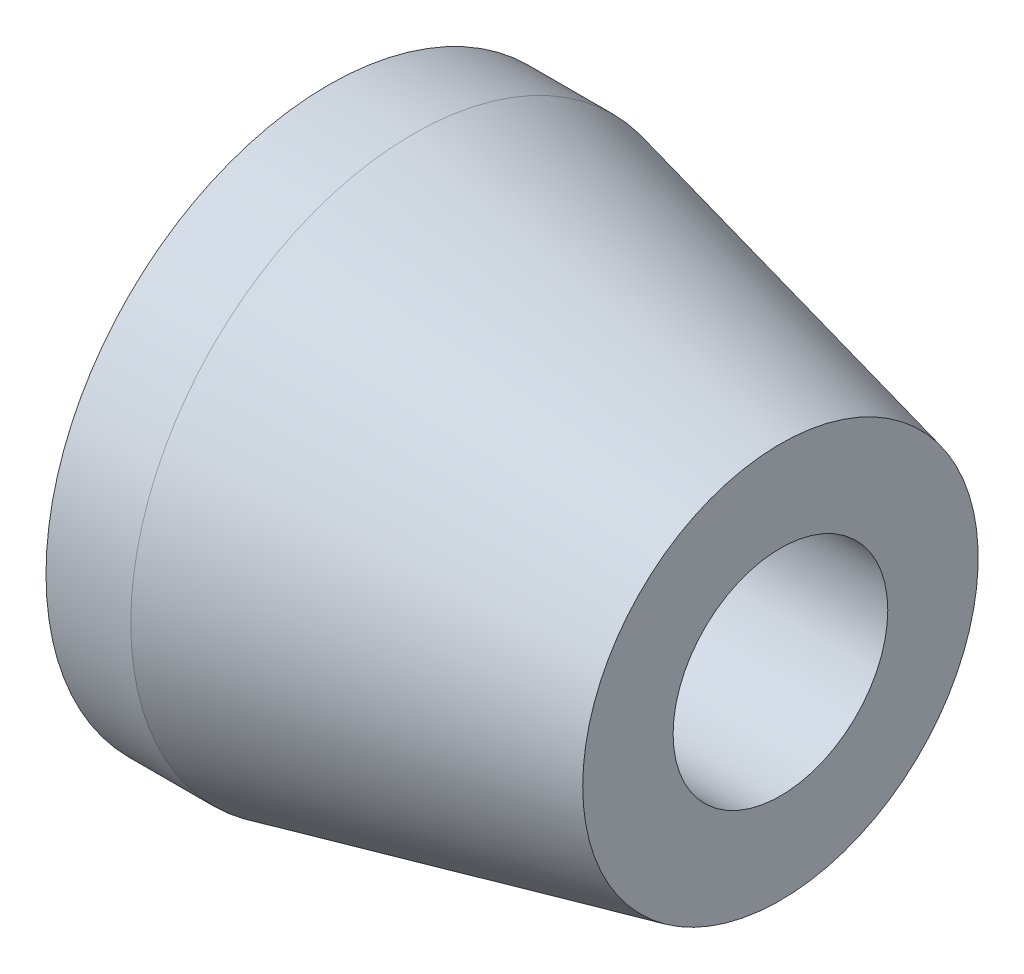
ISO-10303-21;
HEADER;
FILE_DESCRIPTION(('STEP AP214'),'2;1');
FILE_NAME('part.step','',(''),(''),'','','');
FILE_SCHEMA(('AUTOMOTIVE_DESIGN { 1 0 10303 214 1 1 1 1 }'));
ENDSEC;
DATA;
#1=APPLICATION_CONTEXT('core data for automotive mechanical design processes');
#2=APPLICATION_PROTOCOL_DEFINITION('international standard','automotive_design',2000,#1);
#3=PRODUCT_CONTEXT('',#1,'mechanical');
#4=PRODUCT('Part','Part','',(#3));
#5=PRODUCT_RELATED_PRODUCT_CATEGORY('part','',(#4));
#6=PRODUCT_DEFINITION_FORMATION('','',#4);
#7=PRODUCT_DEFINITION_CONTEXT('part definition',#1,'design');
#8=PRODUCT_DEFINITION('design','',#6,#7);
#9=PRODUCT_DEFINITION_SHAPE('','',#8);
#10=(LENGTH_UNIT() NAMED_UNIT(*) SI_UNIT(.MILLI.,.METRE.));
#11=(NAMED_UNIT(*) PLANE_ANGLE_UNIT() SI_UNIT($,.RADIAN.));
#12=(NAMED_UNIT(*) SI_UNIT($,.STERADIAN.) SOLID_ANGLE_UNIT());
#13=UNCERTAINTY_MEASURE_WITH_UNIT(LENGTH_MEASURE(1.E-05),#10,'distance_accuracy_value','');
#14=(GEOMETRIC_REPRESENTATION_CONTEXT(3) GLOBAL_UNCERTAINTY_ASSIGNED_CONTEXT((#13)) GLOBAL_UNIT_ASSIGNED_CONTEXT((#10,
#11,#12)) REPRESENTATION_CONTEXT('',''));
#15=CARTESIAN_POINT('',(0.,0.,0.));
#16=DIRECTION('',(0.,0.,1.));
#17=DIRECTION('',(1.,0.,0.));
#18=AXIS2_PLACEMENT_3D('',#15,#16,#17);
#19=CARTESIAN_POINT('',(16.,0.,0.));
#20=DIRECTION('',(-1.,0.,0.));
#21=DIRECTION('',(0.,0.,1.));
#22=AXIS2_PLACEMENT_3D('',#19,#20,#21);
#23=CYLINDRICAL_SURFACE('',#22,3.8);
#24=CARTESIAN_POINT('',(16.,0.,0.));
#25=DIRECTION('',(-1.,0.,0.));
#26=DIRECTION('',(0.,0.,1.));
#27=AXIS2_PLACEMENT_3D('',#24,#25,#26);
#28=CIRCLE('',#27,3.8);
#29=CARTESIAN_POINT('',(16.,0.,3.8));
#30=VERTEX_POINT('',#29);
#31=EDGE_CURVE('E57',#30,#30,#28,.T.);
#32=ORIENTED_EDGE('',*,*,#31,.F.);
#33=EDGE_LOOP('',(#32));
#34=FACE_BOUND('',#33,.T.);
#35=CARTESIAN_POINT('',(2.,0.,0.));
#36=DIRECTION('',(-1.,0.,0.));
#37=DIRECTION('',(0.,0.,1.));
#38=AXIS2_PLACEMENT_3D('',#35,#36,#37);
#39=CIRCLE('',#38,3.8);
#40=CARTESIAN_POINT('',(2.,0.,3.8));
#41=VERTEX_POINT('',#40);
#42=EDGE_CURVE('E43',#41,#41,#39,.F.);
#43=ORIENTED_EDGE('',*,*,#42,.F.);
#44=EDGE_LOOP('',(#43));
#45=FACE_BOUND('',#44,.T.);
#46=ADVANCED_FACE('F39',(#34,#45),#23,.F.);
#47=CARTESIAN_POINT('',(0.,0.,0.));
#48=DIRECTION('',(1.,0.,0.));
#49=DIRECTION('',(0.,0.,-1.));
#50=AXIS2_PLACEMENT_3D('',#47,#48,#49);
#51=PLANE('',#50);
#52=CARTESIAN_POINT('',(0.,0.,0.));
#53=DIRECTION('',(-1.,0.,0.));
#54=DIRECTION('',(0.,0.,1.));
#55=AXIS2_PLACEMENT_3D('',#52,#53,#54);
#56=CIRCLE('',#55,6.5);
#57=CARTESIAN_POINT('',(0.,0.,6.5));
#58=VERTEX_POINT('',#57);
#59=EDGE_CURVE('E56',#58,#58,#56,.T.);
#60=ORIENTED_EDGE('',*,*,#59,.F.);
#61=EDGE_LOOP('',(#60));
#62=FACE_BOUND('',#61,.T.);
#63=CARTESIAN_POINT('',(0.,0.,0.));
#64=DIRECTION('',(-1.,0.,0.));
#65=DIRECTION('',(0.,0.,1.));
#66=AXIS2_PLACEMENT_3D('',#63,#64,#65);
#67=CIRCLE('',#66,10.);
#68=CARTESIAN_POINT('',(0.,0.,10.));
#69=VERTEX_POINT('',#68);
#70=EDGE_CURVE('E10',#69,#69,#67,.T.);
#71=ORIENTED_EDGE('',*,*,#70,.T.);
#72=EDGE_LOOP('',(#71));
#73=FACE_BOUND('',#72,.T.);
#74=ADVANCED_FACE('F41',(#62,#73),#51,.F.);
#75=CARTESIAN_POINT('',(-1000.,0.,0.));
#76=DIRECTION('',(-1.,0.,0.));
#77=DIRECTION('',(0.,0.,1.));
#78=AXIS2_PLACEMENT_3D('',#75,#76,#77);
#79=CYLINDRICAL_SURFACE('',#78,10.);
#80=ORIENTED_EDGE('',*,*,#70,.F.);
#81=EDGE_LOOP('',(#80));
#82=FACE_BOUND('',#81,.T.);
#83=CARTESIAN_POINT('',(2.99999999999989,0.,0.));
#84=DIRECTION('',(-1.,0.,0.));
#85=DIRECTION('',(0.,0.,1.));
#86=AXIS2_PLACEMENT_3D('',#83,#84,#85);
#87=CIRCLE('',#86,10.);
#88=CARTESIAN_POINT('',(2.99999999999989,0.,10.));
#89=VERTEX_POINT('',#88);
#90=EDGE_CURVE('E50',#89,#89,#87,.T.);
#91=ORIENTED_EDGE('',*,*,#90,.T.);
#92=EDGE_LOOP('',(#91));
#93=FACE_BOUND('',#92,.T.);
#94=ADVANCED_FACE('F77',(#82,#93),#79,.T.);
#95=CARTESIAN_POINT('',(16.,0.,0.));
#96=DIRECTION('',(-1.,0.,0.));
#97=DIRECTION('',(0.,0.,1.));
#98=AXIS2_PLACEMENT_3D('',#95,#96,#97);
#99=CONICAL_SURFACE('',#98,7.,0.226798848053884);
#100=ORIENTED_EDGE('',*,*,#90,.F.);
#101=EDGE_LOOP('',(#100));
#102=FACE_BOUND('',#101,.T.);
#103=CARTESIAN_POINT('',(16.,0.,0.));
#104=DIRECTION('',(-1.,0.,0.));
#105=DIRECTION('',(0.,0.,1.));
#106=AXIS2_PLACEMENT_3D('',#103,#104,#105);
#107=CIRCLE('',#106,7.);
#108=CARTESIAN_POINT('',(16.,0.,7.));
#109=VERTEX_POINT('',#108);
#110=EDGE_CURVE('E51',#109,#109,#107,.T.);
#111=ORIENTED_EDGE('',*,*,#110,.T.);
#112=EDGE_LOOP('',(#111));
#113=FACE_BOUND('',#112,.T.);
#114=ADVANCED_FACE('F87',(#102,#113),#99,.T.);
#115=CARTESIAN_POINT('',(16.,7.,0.));
#116=DIRECTION('',(-1.,0.,0.));
#117=DIRECTION('',(0.,0.,1.));
#118=AXIS2_PLACEMENT_3D('',#115,#116,#117);
#119=PLANE('',#118);
#120=ORIENTED_EDGE('',*,*,#31,.T.);
#121=EDGE_LOOP('',(#120));
#122=FACE_BOUND('',#121,.T.);
#123=ORIENTED_EDGE('',*,*,#110,.F.);
#124=EDGE_LOOP('',(#123));
#125=FACE_BOUND('',#124,.T.);
#126=ADVANCED_FACE('F85',(#122,#125),#119,.F.);
#127=CARTESIAN_POINT('',(2.,0.,0.));
#128=DIRECTION('',(-1.,0.,0.));
#129=DIRECTION('',(0.,0.,1.));
#130=AXIS2_PLACEMENT_3D('',#127,#128,#129);
#131=PLANE('',#130);
#132=CARTESIAN_POINT('',(2.,0.,0.));
#133=DIRECTION('',(-1.,0.,0.));
#134=DIRECTION('',(0.,0.,1.));
#135=AXIS2_PLACEMENT_3D('',#132,#133,#134);
#136=CIRCLE('',#135,6.5);
#137=CARTESIAN_POINT('',(2.,0.,6.5));
#138=VERTEX_POINT('',#137);
#139=EDGE_CURVE('E65',#138,#138,#136,.T.);
#140=ORIENTED_EDGE('',*,*,#139,.T.);
#141=EDGE_LOOP('',(#140));
#142=FACE_BOUND('',#141,.T.);
#143=ORIENTED_EDGE('',*,*,#42,.T.);
#144=EDGE_LOOP('',(#143));
#145=FACE_BOUND('',#144,.T.);
#146=ADVANCED_FACE('F68',(#142,#145),#131,.T.);
#147=CARTESIAN_POINT('',(2.,0.,0.));
#148=DIRECTION('',(-1.,0.,0.));
#149=DIRECTION('',(0.,0.,1.));
#150=AXIS2_PLACEMENT_3D('',#147,#148,#149);
#151=CYLINDRICAL_SURFACE('',#150,6.5);
#152=ORIENTED_EDGE('',*,*,#139,.F.);
#153=EDGE_LOOP('',(#152));
#154=FACE_BOUND('',#153,.T.);
#155=ORIENTED_EDGE('',*,*,#59,.T.);
#156=EDGE_LOOP('',(#155));
#157=FACE_BOUND('',#156,.T.);
#158=ADVANCED_FACE('F84',(#154,#157),#151,.F.);
#159=CLOSED_SHELL('',(#46,#74,#94,#114,#126,#146,#158));
#160=MANIFOLD_SOLID_BREP('B2',#159);
#161=ADVANCED_BREP_SHAPE_REPRESENTATION('',(#18,#160),#14);
#162=SHAPE_DEFINITION_REPRESENTATION(#9,#161);
ENDSEC;
END-ISO-10303-21;
